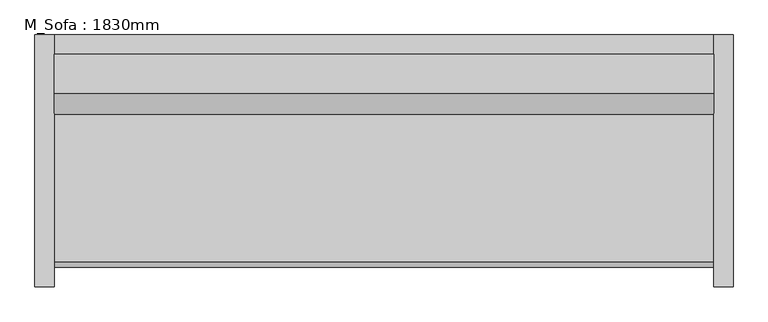
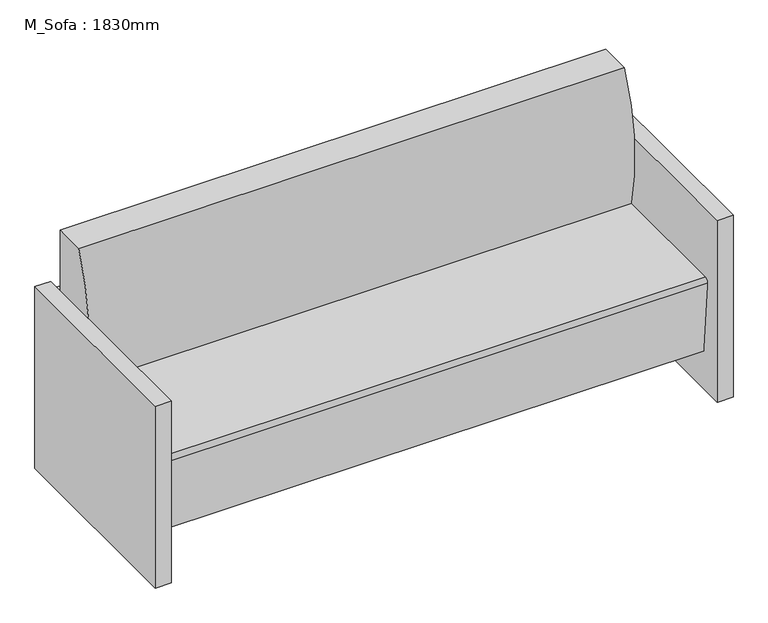
"""IFC4 building model written with IfcOpenShell, lengths in millimetres: furniture geometry, M_Sofa : 1830mm."""

from ifc_helpers import new_model, si_unit, point, frame, frame_2d, origin, origin_with_axes, place, context, project, spatial, polyline, circle_curve, trimmed, segment, composite_curve, outline, extrude, source, transform, mapped, element, save


def m_sofa_1830mm_f9e8a66b(model_context):
    return source(origin(), model_context, "Body", "SweptSolid", [
        extrude(outline(polyline([(-793.8295082, 425.5540984), (-793.8295082, 476.3540984), (934.5704918, 476.3540984), (934.5704918, 425.5540984), (-793.8295082, 425.5540984)])), frame((0.0, 0.0, 457.2), z_axis=(0.0, 0.0, 1.0), x_axis=(1.0, 0.0, 0.0)), (0.0, 0.0, 1.0), 127.0),
        extrude(outline(polyline([(-793.8295082, 425.5540984), (-793.8295082, 476.3540984), (934.5704918, 476.3540984), (934.5704918, 425.5540984), (-793.8295082, 425.5540984)])), frame((0.0, 0.0, 266.7), z_axis=(0.0, 0.0, 1.0), x_axis=(1.0, 0.0, 0.0)), (0.0, 0.0, 1.0), 127.0),
        extrude(outline(polyline([(-793.8295082, 425.5540984), (-793.8295082, 476.3540984), (934.5704918, 476.3540984), (934.5704918, 425.5540984), (-793.8295082, 425.5540984)])), frame((0.0, 0.0, 76.2), z_axis=(0.0, 0.0, 1.0), x_axis=(1.0, 0.0, 0.0)), (0.0, 0.0, 1.0), 127.0),
        extrude(outline(composite_curve([segment(trimmed(circle_curve(frame_2d((926.517198, 542.5300036)), 660.4), [point((286.1764935, 381.0))], [point((323.9540984, 812.8))], False, "CARTESIAN"), True, "CONTINUOUS"), segment(polyline([(323.9540984, 812.8), (425.5540984, 812.8), (425.5540984, 127.9665467), (-111.108343, 127.9665467), (-132.0379563, 367.1931221)]), True, "CONTINUOUS"), segment(trimmed(circle_curve(frame_2d((-119.3862837, 368.3)), 12.7), [point((-132.0379563, 367.1931221))], [point((-119.3862837, 381.0))], False, "CARTESIAN"), True, "CONTINUOUS"), segment(polyline([(-119.3862837, 381.0), (286.1764935, 381.0)]), True, "CONTINUOUS")], self_intersect=False)), frame((-793.8295082, 0.0, 0.0), z_axis=(1.0, 0.0, 0.0), x_axis=(0.0, 1.0, 0.0)), (0.0, 0.0, 1.0), 1728.4),
        extrude(outline(polyline([(-793.8295082, 476.3540984), (-793.8295082, -184.0459016), (-844.6295082, -184.0459016), (-844.6295082, 476.3540984), (-793.8295082, 476.3540984)])), origin_with_axes(), (0.0, 0.0, 1.0), 609.6),
        extrude(outline(polyline([(985.3704918, 476.3540984), (985.3704918, -184.0459016), (934.5704918, -184.0459016), (934.5704918, 476.3540984), (985.3704918, 476.3540984)])), origin_with_axes(), (0.0, 0.0, 1.0), 609.6),
    ])


if __name__ == "__main__":
    model = new_model("IFC4")
    model_context = context("Model", 3, world=origin())
    ifc_project = project(units=[si_unit("LENGTHUNIT", "METRE", prefix="MILLI")], contexts=[model_context])
    site = spatial("IfcSite", under=ifc_project)
    building = spatial("IfcBuilding", under=site)
    placement = place(None, origin())
    m_sofa_1830mm_shape = m_sofa_1830mm_f9e8a66b(model_context)
    element("IfcFurniture", 1, ObjectType="M_Sofa : 1830mm", at=placement, inside=building, context=model_context, shape_type="MappedRepresentation", body=[
        mapped(m_sofa_1830mm_shape, transform((0.0, 0.0, 0.0), x_axis=(1.0, 0.0, 0.0), y_axis=(0.0, 1.0, 0.0), z_axis=(0.0, 0.0, 1.0))),
    ])
    save(model, "model.ifc")

# Revit data of these elements
# Type "M_Sofa : 1830mm"
#   Width = 6' - 0.04724"
#   Seat Material = Linen, Beige
#   Frame Material = Cherry
#   Default Elevation = 0
# Element 1 (IfcFurniture, "M_Sofa : 1830mm")
#   Materials on its faces: "Cherry", "Linen, Beige"
# Materials
#   "Linen, Beige": class "Textile", colour RGB 249 239 230, transparency 0, Description = "Linen, beige", Cost = 0
#   "Cherry": class "Wood", colour RGB 154 107 61, transparency 0, Description = "Prunus Serotina", Cost = 0
